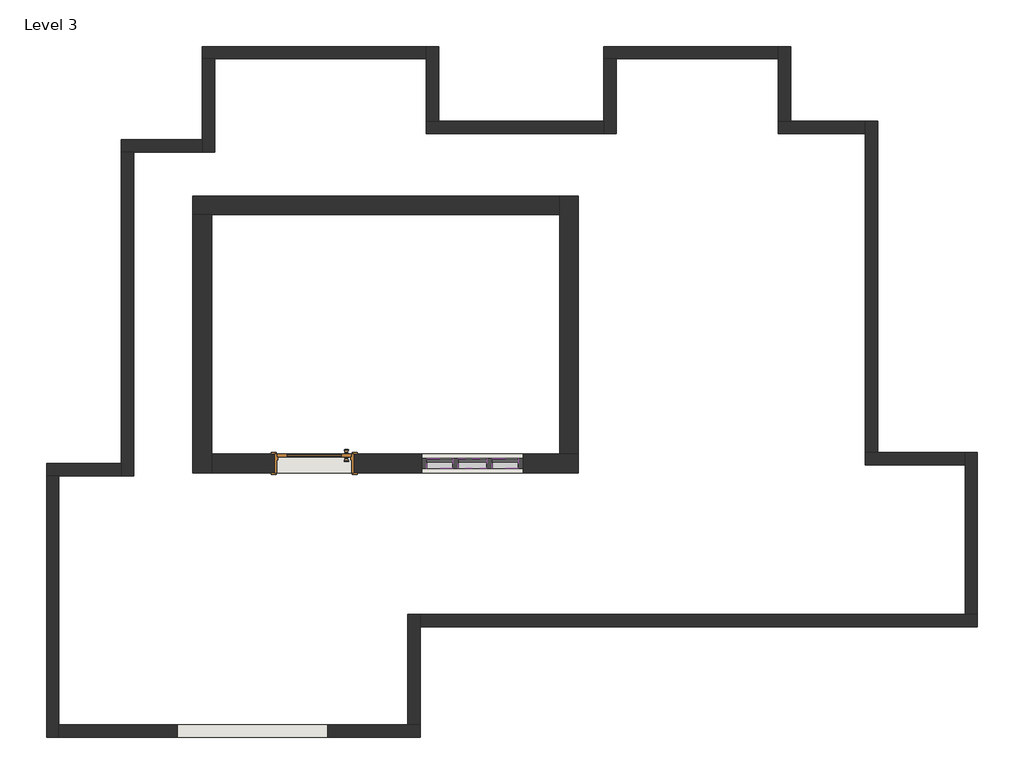
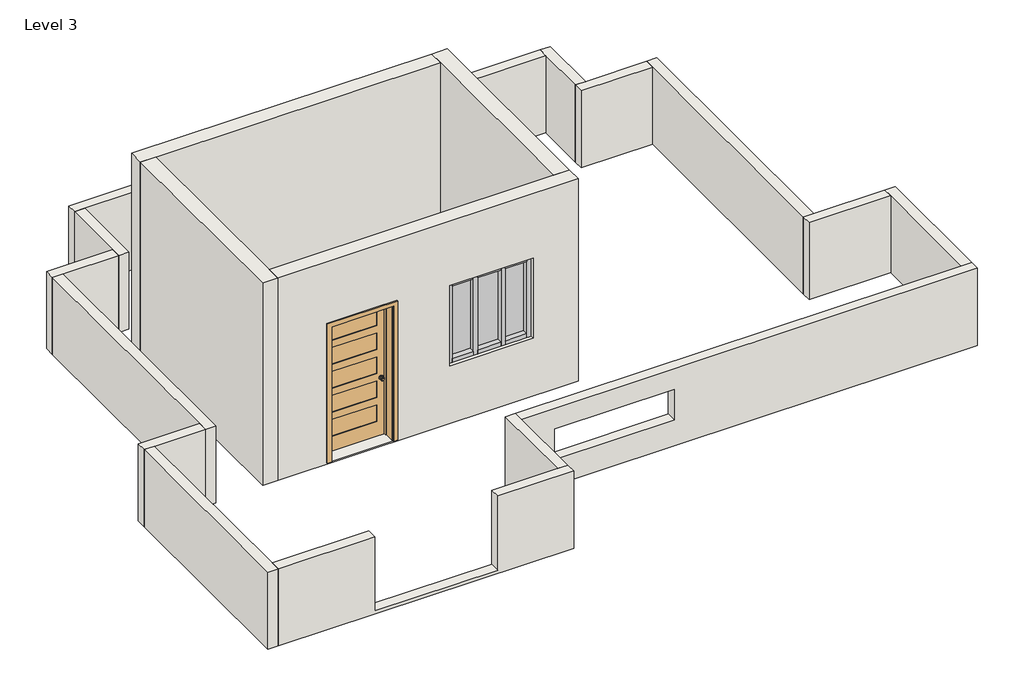
# One storey: 22 walls, 10 members, 3 plates, 1 door.
"""IFC4 building model written with IfcOpenShell, lengths in millimetres."""

from ifc_helpers import new_model, si_unit, origin, place, context, project, spatial, faceted_brep, transform, mapped, element, save
from components import door_e6f20f03, member_91b02dc0, member_4918008d, member_2b44a902, member_ab7d1daf, system_panel_glazed_3c18516d, system_panel_glazed_6a35409e

model = new_model("IFC4")

# Units and contexts
model_context = context("Model", 3, world=origin())
ifc_project = project(units=[si_unit("LENGTHUNIT", "METRE", prefix="MILLI")], contexts=[model_context])

# Site, building, storey
site = spatial("IfcSite", under=ifc_project)
building = spatial("IfcBuilding", under=site)
storey = spatial("IfcBuildingStorey", under=building, Name="Level 3", Elevation=3810.0)

# Door
placement = place(None, origin())
door_shape = door_e6f20f03(model_context)
element("IfcDoor", 1, ObjectType="Door-Interior-Single-5_Panel_Vert-Wood : 3'6\" x 7'", at=placement, inside=storey, context=model_context, shape_type="MappedRepresentation", body=[
    mapped(door_shape, transform((-3850.3928023, 4085.9707931, 3835.4), x_axis=(-1.0, 0.0, 0.0), y_axis=(0.0, -1.0, 0.0), z_axis=(0.0, 0.0, 1.0))),
])

# Members
member_shape = member_91b02dc0(model_context)
element("IfcMember", 2, ObjectType="Rectangular Mullion : 2.5\" x 5\" rectangular", at=placement, inside=storey, context=model_context, shape_type="MappedRepresentation", body=[
    mapped(member_shape, transform((-1355.7364068, 4082.7957931, 5994.4), x_axis=(0.0, 0.0, 1.0), y_axis=(0.0, -1.0, 0.0), z_axis=(1.0, 0.0, 0.0))),
])
element("IfcMember", 3, ObjectType="Rectangular Mullion : 2.5\" x 5\" rectangular", at=placement, inside=storey, context=model_context, shape_type="MappedRepresentation", body=[
    mapped(member_shape, transform((-2153.7197401, 4082.7957931, 5994.4), x_axis=(0.0, 0.0, 1.0), y_axis=(0.0, -1.0, 0.0), z_axis=(1.0, 0.0, 0.0))),
])
element("IfcMember", 4, ObjectType="Rectangular Mullion : 2.5\" x 5\" rectangular", at=placement, inside=storey, context=model_context, shape_type="MappedRepresentation", body=[
    mapped(member_shape, transform((-2473.3364068, 4082.7957931, 4724.4), x_axis=(0.0, 0.0, -1.0), y_axis=(0.0, -1.0, 0.0), z_axis=(-1.0, 0.0, 0.0))),
])
element("IfcMember", 5, ObjectType="Rectangular Mullion : 2.5\" x 5\" rectangular", at=placement, inside=storey, context=model_context, shape_type="MappedRepresentation", body=[
    mapped(member_shape, transform((-1675.3530735, 4082.7957931, 4724.4), x_axis=(0.0, 0.0, -1.0), y_axis=(0.0, -1.0, 0.0), z_axis=(-1.0, 0.0, 0.0))),
])
member_2_shape = member_4918008d(model_context)
element("IfcMember", 6, ObjectType="Rectangular Mullion : 2.5\" x 5\" rectangular", at=placement, inside=storey, context=model_context, shape_type="MappedRepresentation", body=[
    mapped(member_2_shape, transform((-2090.2197401, 4082.7957931, 4724.4), x_axis=(0.0, 0.0, -1.0), y_axis=(0.0, -1.0, 0.0), z_axis=(-1.0, 0.0, 0.0))),
])
element("IfcMember", 7, ObjectType="Rectangular Mullion : 2.5\" x 5\" rectangular", at=placement, inside=storey, context=model_context, shape_type="MappedRepresentation", body=[
    mapped(member_2_shape, transform((-1738.8530735, 4082.7957931, 5994.4), x_axis=(0.0, 0.0, 1.0), y_axis=(0.0, -1.0, 0.0), z_axis=(1.0, 0.0, 0.0))),
])
member_3_shape = member_2b44a902(model_context)
element("IfcMember", 8, ObjectType="Rectangular Mullion : 2.5\" x 5\" rectangular", at=placement, inside=storey, context=model_context, shape_type="MappedRepresentation", body=[
    mapped(member_3_shape, transform((-2121.9697401, 4082.7957931, 4724.4), x_axis=(1.0, 0.0, 0.0), y_axis=(0.0, -1.0, 0.0), z_axis=(0.0, 0.0, -1.0))),
])
element("IfcMember", 9, ObjectType="Rectangular Mullion : 2.5\" x 5\" rectangular", at=placement, inside=storey, context=model_context, shape_type="MappedRepresentation", body=[
    mapped(member_3_shape, transform((-1707.1030735, 4082.7957931, 4724.4), x_axis=(1.0, 0.0, 0.0), y_axis=(0.0, -1.0, 0.0), z_axis=(0.0, 0.0, -1.0))),
])
member_4_shape = member_ab7d1daf(model_context)
element("IfcMember", 10, ObjectType="Rectangular Mullion : 2.5\" x 5\" rectangular", at=placement, inside=storey, context=model_context, shape_type="MappedRepresentation", body=[
    mapped(member_4_shape, transform((-2536.8364068, 4082.7957931, 5994.4), x_axis=(-1.0, 0.0, 0.0), y_axis=(0.0, -1.0, 0.0), z_axis=(0.0, 0.0, 1.0))),
])
element("IfcMember", 11, ObjectType="Rectangular Mullion : 2.5\" x 5\" rectangular", at=placement, inside=storey, context=model_context, shape_type="MappedRepresentation", body=[
    mapped(member_4_shape, transform((-1292.2364068, 4082.7957931, 4724.4), x_axis=(1.0, 0.0, 0.0), y_axis=(0.0, -1.0, 0.0), z_axis=(0.0, 0.0, -1.0))),
])

# Plates
system_panel_glazed_shape = system_panel_glazed_3c18516d(model_context)
element("IfcPlate", 12, ObjectType="System Panel : Glazed", at=placement, inside=storey, context=model_context, shape_type="MappedRepresentation", body=[
    mapped(system_panel_glazed_shape, transform((-2313.5280735, 4082.7957931, 4787.9), x_axis=(1.0, 0.0, 0.0), y_axis=(0.0, 1.0, 0.0), z_axis=(0.0, 0.0, 1.0))),
])
element("IfcPlate", 13, ObjectType="System Panel : Glazed", at=placement, inside=storey, context=model_context, shape_type="MappedRepresentation", body=[
    mapped(system_panel_glazed_shape, transform((-1515.5447401, 4082.7957931, 4787.9), x_axis=(1.0, 0.0, 0.0), y_axis=(0.0, 1.0, 0.0), z_axis=(0.0, 0.0, 1.0))),
])
system_panel_glazed_2_shape = system_panel_glazed_6a35409e(model_context)
element("IfcPlate", 14, ObjectType="System Panel : Glazed", at=placement, inside=storey, context=model_context, shape_type="MappedRepresentation", body=[
    mapped(system_panel_glazed_2_shape, transform((-1914.5364068, 4082.7957931, 4787.9), x_axis=(1.0, 0.0, 0.0), y_axis=(0.0, 1.0, 0.0), z_axis=(0.0, 0.0, 1.0))),
])

# Walls
element("IfcWall", 15, ObjectType="6\"", at=placement, inside=storey, context=model_context, shape_type="Brep", body=[
    faceted_brep([(-6974.5928023, 729.9957931, 3810.0), (-2554.9928023, 729.9957931, 3810.0), (-2554.9928023, 729.9957931, 5029.2), (-3687.4832719, 729.9957931, 5029.2), (-3687.4832719, 729.9957931, 3857.2016305), (-5526.7928023, 729.9957931, 3857.2016305), (-5526.7928023, 729.9957931, 5029.2), (-6974.5928023, 729.9957931, 5029.2), (-2554.9928023, 882.3957931, 3810.0), (-2707.3928023, 882.3957931, 3810.0), (-6974.5928023, 882.3957931, 3810.0), (-6974.5928023, 882.3957931, 5029.2), (-5526.7928023, 882.3957931, 5029.2), (-5526.7928023, 882.3957931, 3857.2016305), (-3687.4832719, 882.3957931, 3857.2016305), (-3687.4832719, 882.3957931, 5029.2), (-2707.3928023, 882.3957931, 5029.2), (-2554.9928023, 882.3957931, 5029.2)], [[[0, 1, 2, 3, 4, 5, 6, 7]], [[8, 9, 10, 11, 12, 13, 14, 15, 16, 17]], [[1, 0, 10, 9, 8]], [[2, 17, 16, 15, 3]], [[11, 7, 6, 12]], [[2, 1, 8, 17]], [[0, 7, 11, 10]], [[4, 14, 13, 5]], [[5, 13, 12, 6]], [[14, 4, 3, 15]]]),
])
element("IfcWall", 16, ObjectType="6\"", at=placement, inside=storey, context=model_context, shape_type="Brep", body=[
    faceted_brep([(-2554.9928023, 882.3957931, 3810.0), (-2554.9928023, 2082.5457931, 3810.0), (-2554.9928023, 2234.9457931, 3810.0), (-2554.9928023, 2234.9457931, 5029.2), (-2554.9928023, 2082.5457931, 5029.2), (-2554.9928023, 882.3957931, 5029.2), (-2707.3928023, 882.3957931, 3810.0), (-2707.3928023, 882.3957931, 5029.2), (-2707.3928023, 2234.9457931, 5029.2), (-2707.3928023, 2234.9457931, 3810.0)], [[[0, 1, 2, 3, 4, 5]], [[6, 7, 8, 9]], [[2, 1, 0, 6, 9]], [[5, 4, 3, 8, 7]], [[0, 5, 7, 6]], [[3, 2, 9, 8]]]),
])
element("IfcWall", 17, ObjectType="6\"", at=placement, inside=storey, context=model_context, shape_type="Brep", body=[
    faceted_brep([(-2554.9928023, 2082.5457931, 3810.0), (4264.9071977, 2082.5457931, 3810.0), (4264.9071977, 2082.5457931, 5029.2), (-2554.9928023, 2082.5457931, 5029.2), (-2057.3683725, 2082.5457931, 4699.0), (-267.0084578, 2082.5457931, 4699.0), (-267.0084578, 2082.5457931, 4216.4), (-2057.3683725, 2082.5457931, 4216.4), (4264.9071977, 2234.9457931, 3810.0), (4112.5071977, 2234.9457931, 3810.0), (-2554.9928023, 2234.9457931, 3810.0), (-2554.9928023, 2234.9457931, 5029.2), (4112.5071977, 2234.9457931, 5029.2), (4264.9071977, 2234.9457931, 5029.2), (-267.0084578, 2234.9457931, 4699.0), (-2057.3683725, 2234.9457931, 4699.0), (-2057.3683725, 2234.9457931, 4216.4), (-267.0084578, 2234.9457931, 4216.4)], [[[0, 1, 2, 3], [4, 5, 6, 7]], [[8, 9, 10, 11, 12, 13], [14, 15, 16, 17]], [[1, 0, 10, 9, 8]], [[3, 2, 13, 12, 11]], [[0, 3, 11, 10]], [[2, 1, 8, 13]], [[4, 15, 14, 5]], [[6, 17, 16, 7]], [[15, 4, 7, 16]], [[5, 14, 17, 6]]]),
])
element("IfcWall", 18, ObjectType="6\"", at=placement, inside=storey, context=model_context, shape_type="Brep", body=[
    faceted_brep([(4264.9071977, 2234.9457931, 3810.0), (4264.9071977, 4216.1457931, 3810.0), (4264.9071977, 4216.1457931, 5029.2), (4264.9071977, 2234.9457931, 5029.2), (4112.5071977, 2234.9457931, 3810.0), (4112.5071977, 2234.9457931, 5029.2), (4112.5071977, 4063.7457931, 5029.2), (4112.5071977, 4216.1457931, 5029.2), (4112.5071977, 4216.1457931, 3810.0), (4112.5071977, 4063.7457931, 3810.0)], [[[0, 1, 2, 3]], [[4, 5, 6, 7, 8, 9]], [[1, 0, 4, 9, 8]], [[3, 2, 7, 6, 5]], [[0, 3, 5, 4]], [[2, 1, 8, 7]]]),
])
element("IfcWall", 19, ObjectType="6\"", at=placement, inside=storey, context=model_context, shape_type="Brep", body=[
    faceted_brep([(4112.5071977, 4216.1457931, 3810.0), (3045.7071977, 4216.1457931, 3810.0), (2893.3071977, 4216.1457931, 3810.0), (2893.3071977, 4216.1457931, 5029.2), (3045.7071977, 4216.1457931, 5029.2), (4112.5071977, 4216.1457931, 5029.2), (4112.5071977, 4063.7457931, 3810.0), (4112.5071977, 4063.7457931, 5029.2), (2893.3071977, 4063.7457931, 5029.2), (2893.3071977, 4063.7457931, 3810.0)], [[[0, 1, 2, 3, 4, 5]], [[6, 7, 8, 9]], [[2, 1, 0, 6, 9]], [[5, 4, 3, 8, 7]], [[0, 5, 7, 6]], [[3, 2, 9, 8]]]),
])
element("IfcWall", 20, ObjectType="6\"", at=placement, inside=storey, context=model_context, shape_type="Brep", body=[
    faceted_brep([(3045.7071977, 4216.1457931, 3810.0), (3045.7071977, 8273.7957931, 3810.0), (3045.7071977, 8273.7957931, 5029.2), (3045.7071977, 4216.1457931, 5029.2), (2893.3071977, 4216.1457931, 3810.0), (2893.3071977, 4216.1457931, 5029.2), (2893.3071977, 8121.3957931, 5029.2), (2893.3071977, 8273.7957931, 5029.2), (2893.3071977, 8273.7957931, 3810.0), (2893.3071977, 8121.3957931, 3810.0)], [[[0, 1, 2, 3]], [[4, 5, 6, 7, 8, 9]], [[1, 0, 4, 9, 8]], [[3, 2, 7, 6, 5]], [[0, 3, 5, 4]], [[2, 1, 8, 7]]]),
])
element("IfcWall", 21, ObjectType="6\"", at=placement, inside=storey, context=model_context, shape_type="Brep", body=[
    faceted_brep([(2893.3071977, 8273.7957931, 3810.0), (1978.9071977, 8273.7957931, 3810.0), (1826.5071977, 8273.7957931, 3810.0), (1826.5071977, 8273.7957931, 5029.2), (1978.9071977, 8273.7957931, 5029.2), (2893.3071977, 8273.7957931, 5029.2), (2893.3071977, 8121.3957931, 3810.0), (2893.3071977, 8121.3957931, 5029.2), (1826.5071977, 8121.3957931, 5029.2), (1826.5071977, 8121.3957931, 3810.0)], [[[0, 1, 2, 3, 4, 5]], [[6, 7, 8, 9]], [[2, 1, 0, 6, 9]], [[5, 4, 3, 8, 7]], [[0, 5, 7, 6]], [[3, 2, 9, 8]]]),
])
element("IfcWall", 22, ObjectType="6\"", at=placement, inside=storey, context=model_context, shape_type="Brep", body=[
    faceted_brep([(1978.9071977, 8273.7957931, 3810.0), (1978.9071977, 9188.1957931, 3810.0), (1978.9071977, 9188.1957931, 5029.2), (1978.9071977, 8273.7957931, 5029.2), (1826.5071977, 8273.7957931, 3810.0), (1826.5071977, 8273.7957931, 5029.2), (1826.5071977, 9035.7957931, 5029.2), (1826.5071977, 9188.1957931, 5029.2), (1826.5071977, 9188.1957931, 3810.0), (1826.5071977, 9035.7957931, 3810.0)], [[[0, 1, 2, 3]], [[4, 5, 6, 7, 8, 9]], [[1, 0, 4, 9, 8]], [[3, 2, 7, 6, 5]], [[0, 3, 5, 4]], [[2, 1, 8, 7]]]),
])
element("IfcWall", 23, ObjectType="6\"", at=placement, inside=storey, context=model_context, shape_type="Brep", body=[
    faceted_brep([(1826.5071977, 9188.1957931, 3810.0), (-307.0928023, 9188.1957931, 3810.0), (-307.0928023, 9188.1957931, 5029.2), (1826.5071977, 9188.1957931, 5029.2), (1826.5071977, 9035.7957931, 3810.0), (1826.5071977, 9035.7957931, 5029.2), (-154.6928023, 9035.7957931, 5029.2), (-307.0928023, 9035.7957931, 5029.2), (-307.0928023, 9035.7957931, 3810.0), (-154.6928023, 9035.7957931, 3810.0)], [[[0, 1, 2, 3]], [[4, 5, 6, 7, 8, 9]], [[1, 0, 4, 9, 8]], [[3, 2, 7, 6, 5]], [[0, 3, 5, 4]], [[2, 1, 8, 7]]]),
])
element("IfcWall", 24, ObjectType="6\"", at=placement, inside=storey, context=model_context, shape_type="Brep", body=[
    faceted_brep([(-307.0928023, 9035.7957931, 3810.0), (-307.0928023, 8273.7957931, 3810.0), (-307.0928023, 8121.3957931, 3810.0), (-307.0928023, 8121.3957931, 5029.2), (-307.0928023, 8273.7957931, 5029.2), (-307.0928023, 9035.7957931, 5029.2), (-154.6928023, 9035.7957931, 3810.0), (-154.6928023, 9035.7957931, 5029.2), (-154.6928023, 8121.3957931, 5029.2), (-154.6928023, 8121.3957931, 3810.0)], [[[0, 1, 2, 3, 4, 5]], [[6, 7, 8, 9]], [[2, 1, 0, 6, 9]], [[5, 4, 3, 8, 7]], [[0, 5, 7, 6]], [[3, 2, 9, 8]]]),
])
element("IfcWall", 25, ObjectType="6\"", at=placement, inside=storey, context=model_context, shape_type="Brep", body=[
    faceted_brep([(-307.0928023, 8273.7957931, 3810.0), (-2326.3928023, 8273.7957931, 3810.0), (-2478.7928023, 8273.7957931, 3810.0), (-2478.7928023, 8273.7957931, 5029.2), (-2326.3928023, 8273.7957931, 5029.2), (-307.0928023, 8273.7957931, 5029.2), (-307.0928023, 8121.3957931, 3810.0), (-307.0928023, 8121.3957931, 5029.2), (-2478.7928023, 8121.3957931, 5029.2), (-2478.7928023, 8121.3957931, 3810.0)], [[[0, 1, 2, 3, 4, 5]], [[6, 7, 8, 9]], [[2, 1, 0, 6, 9]], [[5, 4, 3, 8, 7]], [[0, 5, 7, 6]], [[3, 2, 9, 8]]]),
])
element("IfcWall", 26, ObjectType="6\"", at=placement, inside=storey, context=model_context, shape_type="Brep", body=[
    faceted_brep([(-2326.3928023, 8273.7957931, 3810.0), (-2326.3928023, 9188.1957931, 3810.0), (-2326.3928023, 9188.1957931, 5029.2), (-2326.3928023, 8273.7957931, 5029.2), (-2478.7928023, 8273.7957931, 3810.0), (-2478.7928023, 8273.7957931, 5029.2), (-2478.7928023, 9035.7957931, 5029.2), (-2478.7928023, 9188.1957931, 5029.2), (-2478.7928023, 9188.1957931, 3810.0), (-2478.7928023, 9035.7957931, 3810.0)], [[[0, 1, 2, 3]], [[4, 5, 6, 7, 8, 9]], [[1, 0, 4, 9, 8]], [[3, 2, 7, 6, 5]], [[0, 3, 5, 4]], [[2, 1, 8, 7]]]),
])
element("IfcWall", 27, ObjectType="6\"", at=placement, inside=storey, context=model_context, shape_type="Brep", body=[
    faceted_brep([(-2478.7928023, 9188.1957931, 3810.0), (-5221.9928023, 9188.1957931, 3810.0), (-5221.9928023, 9188.1957931, 5029.2), (-2478.7928023, 9188.1957931, 5029.2), (-2478.7928023, 9035.7957931, 3810.0), (-2478.7928023, 9035.7957931, 5029.2), (-5069.5928023, 9035.7957931, 5029.2), (-5221.9928023, 9035.7957931, 5029.2), (-5221.9928023, 9035.7957931, 3810.0), (-5069.5928023, 9035.7957931, 3810.0)], [[[0, 1, 2, 3]], [[4, 5, 6, 7, 8, 9]], [[1, 0, 4, 9, 8]], [[3, 2, 7, 6, 5]], [[0, 3, 5, 4]], [[2, 1, 8, 7]]]),
])
element("IfcWall", 28, ObjectType="6\"", at=placement, inside=storey, context=model_context, shape_type="Brep", body=[
    faceted_brep([(-5221.9928023, 9035.7957931, 3810.0), (-5221.9928023, 8045.1957931, 3810.0), (-5221.9928023, 7892.7957931, 3810.0), (-5221.9928023, 7892.7957931, 5029.2), (-5221.9928023, 8045.1957931, 5029.2), (-5221.9928023, 9035.7957931, 5029.2), (-5069.5928023, 9035.7957931, 3810.0), (-5069.5928023, 9035.7957931, 5029.2), (-5069.5928023, 7892.7957931, 5029.2), (-5069.5928023, 7892.7957931, 3810.0)], [[[0, 1, 2, 3, 4, 5]], [[6, 7, 8, 9]], [[2, 1, 0, 6, 9]], [[5, 4, 3, 8, 7]], [[0, 5, 7, 6]], [[3, 2, 9, 8]]]),
])
element("IfcWall", 29, ObjectType="6\"", at=placement, inside=storey, context=model_context, shape_type="Brep", body=[
    faceted_brep([(-5221.9928023, 8045.1957931, 3810.0), (-6212.5928023, 8045.1957931, 3810.0), (-6212.5928023, 8045.1957931, 5029.2), (-5221.9928023, 8045.1957931, 5029.2), (-5221.9928023, 7892.7957931, 3810.0), (-5221.9928023, 7892.7957931, 5029.2), (-6060.1928023, 7892.7957931, 5029.2), (-6212.5928023, 7892.7957931, 5029.2), (-6212.5928023, 7892.7957931, 3810.0), (-6060.1928023, 7892.7957931, 3810.0)], [[[0, 1, 2, 3]], [[4, 5, 6, 7, 8, 9]], [[1, 0, 4, 9, 8]], [[3, 2, 7, 6, 5]], [[0, 3, 5, 4]], [[2, 1, 8, 7]]]),
])
element("IfcWall", 30, ObjectType="6\"", at=placement, inside=storey, context=model_context, shape_type="Brep", body=[
    faceted_brep([(-6212.5928023, 7892.7957931, 3810.0), (-6212.5928023, 4082.7957931, 3810.0), (-6212.5928023, 3930.3957931, 3810.0), (-6212.5928023, 3930.3957931, 5029.2), (-6212.5928023, 4082.7957931, 5029.2), (-6212.5928023, 7892.7957931, 5029.2), (-6060.1928023, 7892.7957931, 3810.0), (-6060.1928023, 7892.7957931, 5029.2), (-6060.1928023, 3930.3957931, 5029.2), (-6060.1928023, 3930.3957931, 3810.0)], [[[0, 1, 2, 3, 4, 5]], [[6, 7, 8, 9]], [[2, 1, 0, 6, 9]], [[5, 4, 3, 8, 7]], [[0, 5, 7, 6]], [[3, 2, 9, 8]]]),
])
element("IfcWall", 31, ObjectType="6\"", at=placement, inside=storey, context=model_context, shape_type="Brep", body=[
    faceted_brep([(-6212.5928023, 4082.7957931, 3810.0), (-7126.9928023, 4082.7957931, 3810.0), (-7126.9928023, 4082.7957931, 5029.2), (-6212.5928023, 4082.7957931, 5029.2), (-6212.5928023, 3930.3957931, 3810.0), (-6212.5928023, 3930.3957931, 5029.2), (-6974.5928023, 3930.3957931, 5029.2), (-7126.9928023, 3930.3957931, 5029.2), (-7126.9928023, 3930.3957931, 3810.0), (-6974.5928023, 3930.3957931, 3810.0)], [[[0, 1, 2, 3]], [[4, 5, 6, 7, 8, 9]], [[1, 0, 4, 9, 8]], [[3, 2, 7, 6, 5]], [[0, 3, 5, 4]], [[2, 1, 8, 7]]]),
])
element("IfcWall", 32, ObjectType="6\"", at=placement, inside=storey, context=model_context, shape_type="Brep", body=[
    faceted_brep([(-7126.9928023, 3930.3957931, 3810.0), (-7126.9928023, 729.9957931, 3810.0), (-7126.9928023, 729.9957931, 5029.2), (-7126.9928023, 3930.3957931, 5029.2), (-6974.5928023, 3930.3957931, 3810.0), (-6974.5928023, 3930.3957931, 5029.2), (-6974.5928023, 882.3957931, 5029.2), (-6974.5928023, 729.9957931, 5029.2), (-6974.5928023, 729.9957931, 3810.0), (-6974.5928023, 882.3957931, 3810.0)], [[[0, 1, 2, 3]], [[4, 5, 6, 7, 8, 9]], [[1, 0, 4, 9, 8]], [[3, 2, 7, 6, 5]], [[0, 3, 5, 4]], [[2, 1, 8, 7]]]),
])
element("IfcWall", 33, ObjectType="9\" wall", at=placement, inside=storey, context=model_context, shape_type="Brep", body=[
    faceted_brep([(-5336.2928023, 7129.6874556, 3810.0), (-5107.6928023, 7129.6874556, 3810.0), (-847.7364068, 7129.6874556, 3810.0), (-847.7364068, 7129.6874556, 7010.4), (-5107.6928023, 7129.6874556, 7010.4), (-5336.2928023, 7129.6874556, 7010.4), (-5336.2928023, 7358.2874556, 3810.0), (-5336.2928023, 7358.2874556, 7010.4), (-847.7364068, 7358.2874556, 7010.4), (-847.7364068, 7358.2874556, 3810.0)], [[[0, 1, 2, 3, 4, 5]], [[6, 7, 8, 9]], [[2, 1, 0, 6, 9]], [[5, 4, 3, 8, 7]], [[0, 5, 7, 6]], [[3, 2, 9, 8]]]),
])
element("IfcWall", 34, ObjectType="9\" wall", at=placement, inside=storey, context=model_context, shape_type="Brep", body=[
    faceted_brep([(-5107.6928023, 3968.4957931, 3810.0), (-5107.6928023, 4197.0957931, 3810.0), (-5107.6928023, 7129.6874556, 3810.0), (-5107.6928023, 7129.6874556, 7010.4), (-5107.6928023, 4197.0957931, 7010.4), (-5107.6928023, 3968.4957931, 7010.4), (-5336.2928023, 3968.4957931, 3810.0), (-5336.2928023, 3968.4957931, 7010.4), (-5336.2928023, 7129.6874556, 7010.4), (-5336.2928023, 7129.6874556, 3810.0)], [[[0, 1, 2, 3, 4, 5]], [[6, 7, 8, 9]], [[2, 1, 0, 6, 9]], [[5, 4, 3, 8, 7]], [[0, 5, 7, 6]], [[3, 2, 9, 8]]]),
])
element("IfcWall", 35, ObjectType="9\" wall", at=placement, inside=storey, context=model_context, shape_type="Brep", body=[
    faceted_brep([(-619.1364068, 4197.0957931, 3810.0), (-847.7364068, 4197.0957931, 3810.0), (-5107.6928023, 4197.0957931, 3810.0), (-5107.6928023, 4197.0957931, 7010.4), (-847.7364068, 4197.0957931, 7010.4), (-619.1364068, 4197.0957931, 7010.4), (-4332.9928023, 4197.0957931, 5994.4), (-4332.9928023, 4197.0957931, 3835.4), (-3367.7928023, 4197.0957931, 3835.4), (-3367.7928023, 4197.0957931, 5994.4), (-2536.8364068, 4197.0957931, 5994.4), (-2536.8364068, 4197.0957931, 4724.4), (-1292.2364068, 4197.0957931, 4724.4), (-1292.2364068, 4197.0957931, 5994.4), (-5107.6928023, 3968.4957931, 3810.0), (-619.1364068, 3968.4957931, 3810.0), (-619.1364068, 3968.4957931, 7010.4), (-5107.6928023, 3968.4957931, 7010.4), (-4332.9928023, 3968.4957931, 3835.4), (-4332.9928023, 3968.4957931, 5994.4), (-3367.7928023, 3968.4957931, 5994.4), (-3367.7928023, 3968.4957931, 3835.4), (-2536.8364068, 3968.4957931, 4724.4), (-2536.8364068, 3968.4957931, 5994.4), (-1292.2364068, 3968.4957931, 5994.4), (-1292.2364068, 3968.4957931, 4724.4)], [[[0, 1, 2, 3, 4, 5], [6, 7, 8, 9], [10, 11, 12, 13]], [[14, 15, 16, 17], [18, 19, 20, 21], [22, 23, 24, 25]], [[2, 1, 0, 15, 14]], [[5, 4, 3, 17, 16]], [[0, 5, 16, 15]], [[3, 2, 14, 17]], [[18, 7, 6, 19]], [[19, 6, 9, 20]], [[8, 21, 20, 9]], [[7, 18, 21, 8]], [[22, 11, 10, 23]], [[23, 10, 13, 24]], [[24, 13, 12, 25]], [[11, 22, 25, 12]]]),
])
element("IfcWall", 36, ObjectType="9\" wall", at=placement, inside=storey, context=model_context, shape_type="Brep", body=[
    faceted_brep([(-847.7364068, 7358.2874556, 3810.0), (-847.7364068, 7129.6874556, 3810.0), (-847.7364068, 4197.0957931, 3810.0), (-847.7364068, 4197.0957931, 7010.4), (-847.7364068, 7129.6874556, 7010.4), (-847.7364068, 7358.2874556, 7010.4), (-619.1364068, 7358.2874556, 3810.0), (-619.1364068, 7358.2874556, 7010.4), (-619.1364068, 4197.0957931, 7010.4), (-619.1364068, 4197.0957931, 3810.0)], [[[0, 1, 2, 3, 4, 5]], [[6, 7, 8, 9]], [[2, 1, 0, 6, 9]], [[5, 4, 3, 8, 7]], [[0, 5, 7, 6]], [[3, 2, 9, 8]]]),
])

save(model, "model.ifc")

# Revit data of these elements
# Type "Door-Interior-Single-5_Panel_Vert-Wood : 3'6\" x 7'"
#   Type Mark = "9"
#   Assembly Code = "C1020300"
#   Analytic Construction = "Wooden"
#   Top Rail = 0' - 4 11/16"
#   Thickness = 0' - 1 3/8"
#   Thermal Resistance (R) = 2.5876 (h·ft²·°F)/BTU
#   Swing Angle [instance default] = 90.00°
#   Stiles = 0' - 4 3/4"
#   Rough Width = 3' - 2"
#   Rough Height = 7' - 1"
#   Intermediate Rail = 0' - 4 1/2"
#   Height = 7' - 0"
#   Width = 3' - 0"
#   Heat Transfer Coefficient (U) = 0.3865 BTU/(h·ft²·°F)
#   Bottom Rail = 0' - 9 1/8"
#   Trim Material = DOOR 1
#   Panel Material = DOOR 1
#   Frame Material = DOOR 1
#   Door Handle Material = Aluminum
#   Visual Light Transmittance = 0
#   Solar Heat Gain Coefficient = 0
#   Wall Closure = (empty or 0)
#   Function = (empty or 0)
# Type "Rectangular Mullion : 2.5\" x 5\" rectangular"
#   built-in parameter 1007304 = 0.416667 (stored number, unit not read)
#   built-in parameter 1007301 = 0.104167 (stored number, unit not read)
#   built-in parameter 1007300 = 0.104167 (stored number, unit not read)
# Type "System Panel : Glazed"
#   Construction Type Id = "GSP4R"
#   Analytic Construction = "1/8 in Pilkington single glazing"
#   Visual Light Transmittance = 0.9
#   Solar Heat Gain Coefficient = 0.86
#   Heat Transfer Coefficient (U) = 1.18115 BTU/(h·ft²·°F)
#   Define Thermal Properties by = 1
# Type "6\""
#   Assembly Code = "B2010"
#   Layers, outside or top first: 0' - 6" "Gypsum Wall Board" (function 1)
# Type "9\" wall"
#   Assembly Code = "B2010"
#   Layers, outside or top first: 0' - 9" "Gypsum Wall Board" (function 1)
# Element 1 (IfcDoor, "Door-Interior-Single-5_Panel_Vert-Wood : 3'6\" x 7'")
#   Swing Angle = 90.00°
#   Phase Created = New Construction
#   Materials on its faces: "DOOR 1", "Aluminum"
# Elements 2, 3, 4, 5, 6, 7, 8, 9, 10, 11 (IfcMember, "Rectangular Mullion : 2.5\" x 5\" rectangular")
#   Phase Created = New Construction
# Elements 12, 13, 14 (IfcPlate, "System Panel : Glazed")
#   Phase Created = New Construction
#   Materials on its faces: "Glass"
# Elements 15, 16, 17, 18, 19, 20, 21, 22, 23, 24, 25, 26, 27, 28, 29, 30, 31, 32 (IfcWall, "6\"")
#   Top Offset = 0' - 0"
#   Base Offset = 0' - 0"
#   Unconnected Height = 4' - 0"
#   wall height = 4' - 0"
#   Phase Created = New Construction
#   Base Constraint = Level 3
#   Materials on its faces: "Gypsum Wall Board"
# Elements 33, 34, 35, 36 (IfcWall, "9\" wall")
#   Top Offset = 0' - 0"
#   Base Offset = 0' - 0"
#   wall height = 10' - 6"
#   Phase Created = New Construction
#   Base Constraint = Level 3
#   Top Constraint = Level 4
#   Materials on its faces: "Gypsum Wall Board"
# Materials
#   "DOOR 1": class "Generic", colour RGB 120 120 120, transparency 0, Cost = 0
#   "Aluminum": class "Metal", colour RGB 247 247 247, transparency 0, Description = "Aluminum 6061", Cost = 0
#   "Gypsum Wall Board": class "Generic", colour RGB 127 127 127, transparency 0, Description = "Gypsum Wall Board", Cost = 0
#   "Glass": class "Glass", colour RGB 0 128 192, transparency 0.75, Description = "Soda Lime Glass", Cost = 0
